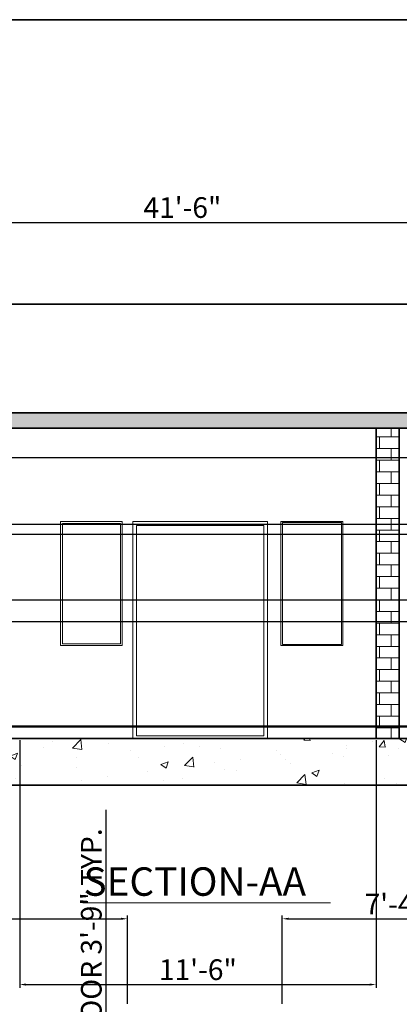
# Model space of a CAD drawing. Units: inches. Extents: x 2257 to 3678, y 834 to 1975.
# Tile 10 of 16: x 3191 to 3338, y 1594 to 1975. Entities that reach past the tile are written whole.
import ezdxf

# ---------------------------------------------------------------- set-up
doc = ezdxf.new("R2010")
doc.units = ezdxf.units.IN
for name, color, linetype, lineweight in [('A-ANNO-DIMS', 2, 'Continuous', 18), ('A-ANNO-TEXT', 7, 'Continuous', 18), ('A-ANNO-TTLB', 7, 'Continuous', 35), ('A-ELEV-DOOR', 3, 'Continuous', 18), ('A-ELEV-GLAZ', 4, 'Continuous', 18), ('A-SECT', 7, 'Continuous', 35), ('A-SECT-BRCK-PATT', 252, 'Continuous', 13), ('A-SECT-CONC-PATT', 252, 'Continuous', 13)]:
    doc.layers.add(name, color=color, linetype=linetype, lineweight=lineweight)
doc.styles.get("Standard").update_dxf_attribs({"font": 'arial.ttf'})
doc.dimstyles.new('ISO-25', dxfattribs={"dimtxt": 8, "dimasz": 2.5, "dimexe": 1.25, "dimexo": 0.625, "dimtad": 1, "dimdec": 0, "dimlunit": 3, "dimtxsty": 'Standard', "dimcen": 2.5, "dimadec": 0, "dimazin": 0, "dimtfac": 1, "dimtdec": 0, "dimtmove": 0, "dimatfit": 3, "dimfxl": 1, "dimarcsym": 0})

# ---------------------------------------------------------------- blocks, each defined once
blk = doc.blocks.new('*D62')
at = {"layer": 'A-ANNO-DIMS', "color": 0, "lineweight": -2, "transparency": 16777216}
for p, q in [((3224.23, 1485.58), (3224.23, 1669.32)), ((3218.11, 1485.58), (3225.48, 1485.58)), ((3224.23, 1443.08), (3224.23, 1483.08)), ((3218.11, 1440.58), (3225.48, 1440.58))]:
    blk.add_line(p, q, dxfattribs=at)
at = {"layer": 'A-ANNO-DIMS', "color": 0, "transparency": 16777216}
for points in [[(3223.82, 1483.08), (3224.65, 1483.08), (3224.23, 1485.58)], [(3223.82, 1443.08), (3224.65, 1443.08), (3224.23, 1440.58)]]:
    blk.add_solid(points, dxfattribs=at)
at = {"layer": 'Defpoints', "color": 0, "transparency": 16777216}
for p in [(3217.48, 1485.58), (3224.23, 1485.58), (3217.48, 1440.58)]:
    blk.add_point(p, dxfattribs=at)
at = {"layer": 'A-ANNO-DIMS', "color": 0, "transparency": 16777216, "insert": (3219.47, 1578.7), "char_height": 8, "attachment_point": 5, "rotation": 90}
blk.add_mtext('REAR BEDROOM DOOR 3\'-9" TYP.', dxfattribs=at)
blk = doc.blocks.new('*D109')
at = {"layer": 'A-ANNO-DIMS', "color": 0, "lineweight": -2, "transparency": 16777216}
for p, q in [((3112.29, 1594.2), (3112.29, 1628.38)), ((3114.79, 1627.13), (3229.89, 1627.13)), ((3232.39, 1594.2), (3232.39, 1628.38))]:
    blk.add_line(p, q, dxfattribs=at)
at = {"layer": 'A-ANNO-DIMS', "color": 0, "transparency": 16777216}
for points in [[(3114.79, 1627.54), (3114.79, 1626.71), (3112.29, 1627.13)], [(3229.89, 1627.54), (3229.89, 1626.71), (3232.39, 1627.13)]]:
    blk.add_solid(points, dxfattribs=at)
at = {"layer": 'Defpoints', "color": 0, "transparency": 16777216}
for p in [(3232.39, 1627.13), (3112.29, 1593.58), (3232.39, 1593.58)]:
    blk.add_point(p, dxfattribs=at)
at = {"layer": 'A-ANNO-DIMS', "color": 0, "transparency": 16777216, "insert": (3172.34, 1631.84), "char_height": 8, "attachment_point": 5}
blk.add_mtext('10\'-0"', dxfattribs=at)
blk = doc.blocks.new('*D110')
at = {"layer": 'A-ANNO-DIMS', "color": 0, "lineweight": -2, "transparency": 16777216}
for p, q in [((3292.39, 1594.2), (3292.39, 1628.38)), ((3294.89, 1627.13), (3377.71, 1627.13)), ((3380.21, 1594.2), (3380.21, 1628.38))]:
    blk.add_line(p, q, dxfattribs=at)
at = {"layer": 'A-ANNO-DIMS', "color": 0, "transparency": 16777216}
for points in [[(3294.89, 1627.54), (3294.89, 1626.71), (3292.39, 1627.13)], [(3377.71, 1627.54), (3377.71, 1626.71), (3380.21, 1627.13)]]:
    blk.add_solid(points, dxfattribs=at)
at = {"layer": 'Defpoints', "color": 0, "transparency": 16777216}
for p in [(3380.21, 1627.13), (3292.39, 1593.58), (3380.21, 1593.58)]:
    blk.add_point(p, dxfattribs=at)
at = {"layer": 'A-ANNO-DIMS', "color": 0, "transparency": 16777216, "insert": (3336.3, 1631.75), "char_height": 8, "attachment_point": 5}
blk.add_mtext('7\'-4"', dxfattribs=at)
blk = doc.blocks.new('*D133')
at = {"layer": 'A-ANNO-DIMS', "color": 0, "lineweight": -2, "transparency": 16777216}
for p, q in [((3004.7, 1865.47), (3004.7, 1897.74)), ((3502.7, 1865.47), (3502.7, 1897.74)), ((3007.2, 1896.49), (3500.2, 1896.49))]:
    blk.add_line(p, q, dxfattribs=at)
at = {"layer": 'A-ANNO-DIMS', "color": 0, "transparency": 16777216}
for points in [[(3007.2, 1896.91), (3007.2, 1896.07), (3004.7, 1896.49)], [(3500.2, 1896.91), (3500.2, 1896.07), (3502.7, 1896.49)]]:
    blk.add_solid(points, dxfattribs=at)
at = {"layer": 'Defpoints', "color": 0, "transparency": 16777216}
for p in [(3502.7, 1896.49), (3004.7, 1864.84), (3502.7, 1864.84)]:
    blk.add_point(p, dxfattribs=at)
at = {"layer": 'A-ANNO-DIMS', "color": 0, "transparency": 16777216, "insert": (3253.7, 1901.2), "char_height": 8, "attachment_point": 5}
blk.add_mtext('41\'-6"', dxfattribs=at)
blk = doc.blocks.new('*D136')
at = {"layer": 'A-ANNO-DIMS', "color": 0, "lineweight": -2, "transparency": 16777216}
for p, q in [((3190.7, 1696.22), (3190.7, 1600.44)), ((3328.7, 1696.22), (3328.7, 1600.44)), ((3193.2, 1601.69), (3326.2, 1601.69))]:
    blk.add_line(p, q, dxfattribs=at)
at = {"layer": 'A-ANNO-DIMS', "color": 0, "transparency": 16777216}
for points in [[(3193.2, 1602.1), (3193.2, 1601.27), (3190.7, 1601.69)], [(3326.2, 1602.1), (3326.2, 1601.27), (3328.7, 1601.69)]]:
    blk.add_solid(points, dxfattribs=at)
at = {"layer": 'Defpoints', "color": 0, "transparency": 16777216}
for p in [(3190.7, 1696.84), (3328.7, 1696.84), (3328.7, 1601.69)]:
    blk.add_point(p, dxfattribs=at)
at = {"layer": 'A-ANNO-DIMS', "color": 0, "transparency": 16777216, "insert": (3259.7, 1606.4), "char_height": 8, "attachment_point": 5}
blk.add_mtext('11\'-6"', dxfattribs=at)
blk = doc.blocks.new('*D145')
at = {"layer": 'A-ANNO-DIMS', "color": 0, "lineweight": -2, "transparency": 16777216}
for p, q in [((3353.28, 1805.46), (2971.8, 1805.46)), ((2973.05, 1782.13), (2973.05, 1802.96)), ((3353.28, 1779.63), (2971.8, 1779.63))]:
    blk.add_line(p, q, dxfattribs=at)
at = {"layer": 'A-ANNO-DIMS', "color": 0, "transparency": 16777216}
for points in [[(2972.63, 1802.96), (2973.47, 1802.96), (2973.05, 1805.46)], [(2972.63, 1782.13), (2973.47, 1782.13), (2973.05, 1779.63)]]:
    blk.add_solid(points, dxfattribs=at)
at = {"layer": 'Defpoints', "color": 0, "transparency": 16777216}
for p in [(2973.05, 1805.46), (3353.91, 1805.46), (3353.91, 1779.63)]:
    blk.add_point(p, dxfattribs=at)
at = {"layer": 'A-ANNO-DIMS', "color": 0, "transparency": 16777216, "insert": (2968.41, 1792.54), "char_height": 8, "attachment_point": 5, "rotation": 90}
blk.add_mtext('2\'-2"', dxfattribs=at)
blk = doc.blocks.new('*D146')
at = {"layer": 'A-ANNO-DIMS', "color": 0, "lineweight": -2, "transparency": 16777216}
for p, q in [((2973.05, 1703.73), (2973.05, 1747.39)), ((3353.28, 1701.23), (2971.8, 1701.23)), ((2973.05, 1696.7), (2973.05, 1701.23)), ((3353.28, 1696.7), (2971.8, 1696.7)), ((2973.05, 1694.2), (2973.05, 1691.7))]:
    blk.add_line(p, q, dxfattribs=at)
at = {"layer": 'A-ANNO-DIMS', "color": 0, "transparency": 16777216}
for points in [[(2972.63, 1703.73), (2973.47, 1703.73), (2973.05, 1701.23)], [(2972.63, 1694.2), (2973.47, 1694.2), (2973.05, 1696.7)]]:
    blk.add_solid(points, dxfattribs=at)
at = {"layer": 'Defpoints', "color": 0, "transparency": 16777216}
for p in [(2973.05, 1701.23), (3353.91, 1701.23), (3353.91, 1696.7)]:
    blk.add_point(p, dxfattribs=at)
at = {"layer": 'A-ANNO-DIMS', "color": 0, "transparency": 16777216, "insert": (2968.29, 1726.81), "char_height": 8, "attachment_point": 5, "rotation": 90}
blk.add_mtext('0\'-4 1/2"', dxfattribs=at)
blk = doc.blocks.new('*D148')
at = {"layer": 'A-ANNO-DIMS', "color": 0, "lineweight": -2, "transparency": 16777216}
for p, q in [((3375.03, 1775.78), (2971.8, 1775.78)), ((2973.05, 1744.52), (2973.05, 1773.28)), ((3375.03, 1742.02), (2971.8, 1742.02))]:
    blk.add_line(p, q, dxfattribs=at)
at = {"layer": 'A-ANNO-DIMS', "color": 0, "transparency": 16777216}
for points in [[(2972.63, 1773.28), (2973.47, 1773.28), (2973.05, 1775.78)], [(2972.63, 1744.52), (2973.47, 1744.52), (2973.05, 1742.02)]]:
    blk.add_solid(points, dxfattribs=at)
at = {"layer": 'Defpoints', "color": 0, "transparency": 16777216}
for p in [(2973.05, 1775.78), (3375.66, 1775.78), (3375.66, 1742.02)]:
    blk.add_point(p, dxfattribs=at)
at = {"layer": 'A-ANNO-DIMS', "color": 0, "transparency": 16777216, "insert": (2968.34, 1758.9), "char_height": 8, "attachment_point": 5, "rotation": 90}
blk.add_mtext('2\'-10"', dxfattribs=at)
blk = doc.blocks.new('*D149')
at = {"layer": 'A-ANNO-DIMS', "color": 0, "lineweight": -2, "transparency": 16777216}
for p, q in [((3417.18, 1750.35), (2971.8, 1750.35)), ((2973.05, 1704.19), (2973.05, 1747.85)), ((3417.18, 1701.69), (2971.8, 1701.69))]:
    blk.add_line(p, q, dxfattribs=at)
at = {"layer": 'A-ANNO-DIMS', "color": 0, "transparency": 16777216}
for points in [[(2972.63, 1747.85), (2973.47, 1747.85), (2973.05, 1750.35)], [(2972.63, 1704.19), (2973.47, 1704.19), (2973.05, 1701.69)]]:
    blk.add_solid(points, dxfattribs=at)
at = {"layer": 'Defpoints', "color": 0, "transparency": 16777216}
for p in [(2973.05, 1750.35), (3417.8, 1750.35), (3417.8, 1701.69)]:
    blk.add_point(p, dxfattribs=at)
at = {"layer": 'A-ANNO-DIMS', "color": 0, "transparency": 16777216, "insert": (2968.29, 1726.02), "char_height": 8, "attachment_point": 5, "rotation": 90}
blk.add_mtext('4\'-0 1/2"', dxfattribs=at)

msp = doc.modelspace()

# ---------------------------------------------------------------- hatches: boundary and pattern name
at = {"layer": 'A-SECT-BRCK-PATT'}
h = msp.add_hatch(dxfattribs=at)
h.set_pattern_fill('BRICK', color=256, scale=0.708661, style=0)
h.paths.add_polyline_path([(3328.7, 1696.84), (3337.7, 1696.84), (3337.7, 1816.84), (3328.7, 1816.84)])
at = {"layer": 'A-SECT-CONC-PATT'}
h = msp.add_hatch(dxfattribs=at)
h.set_pattern_fill('AR-CONC', color=256, scale=0.035, style=0)
h.paths.add_polyline_path([(3004.7, 1816.84), (3502.7, 1816.84), (3502.7, 1822.84), (3004.7, 1822.84)])
h = msp.add_hatch(dxfattribs=at)
h.set_pattern_fill('AR-CONC', color=256, scale=0.16, style=0)
h.paths.add_polyline_path([(3004.7, 1678.84), (3502.7, 1678.84), (3502.7, 1696.84), (3004.7, 1696.84)])

# ---------------------------------------------------------------- linework, layer by layer
at = {"layer": 'A-ANNO-TEXT'}
msp.add_line((3215.12, 1633.34), (3311.06, 1633.34), dxfattribs=at)
at = {"layer": 'A-ANNO-TTLB'}
msp.add_lwpolyline([(2257.38, 1974.9), (3677.96, 1974.9), (3677.96, 849.42), (2257.38, 849.42)], close=True, dxfattribs=at)
at = {"layer": 'A-ELEV-DOOR'}
for p, q in [((3234.47, 1780.84), (3234.47, 1696.84)), ((3286.61, 1780.84), (3234.47, 1780.84)), ((3286.61, 1780.84), (3286.61, 1696.84))]:
    msp.add_line(p, q, dxfattribs=at)
msp.add_lwpolyline([(3235.96, 1779.24), (3285.29, 1779.24), (3285.29, 1697.9), (3235.96, 1697.9)], close=True, dxfattribs=at)
at = {"layer": 'A-ELEV-GLAZ'}
for p, q in [((3206.45, 1780.84), (3206.45, 1732.84)), ((3230.45, 1780.84), (3206.45, 1780.84)), ((3230.45, 1780.84), (3230.45, 1732.84)), ((3291.87, 1780.84), (3291.87, 1732.84)), ((3315.87, 1780.84), (3291.87, 1780.84)), ((3315.87, 1780.84), (3315.87, 1732.84)), ((3230.45, 1732.84), (3206.45, 1732.84)), ((3315.87, 1732.84), (3291.87, 1732.84))]:
    msp.add_line(p, q, dxfattribs=at)
for points in [[(3207.28, 1779.99), (3229.75, 1779.99), (3229.75, 1733.49), (3207.28, 1733.49)], [(3292.45, 1780.37), (3315.31, 1780.37), (3315.31, 1733.21), (3292.45, 1733.21)]]:
    msp.add_lwpolyline(points, close=True, dxfattribs=at)
at = {"layer": 'A-SECT'}
for p, q in [((3502.7, 1864.84), (3004.7, 1864.84)), ((3502.7, 1822.84), (3004.7, 1822.84)), ((3196.31, 1816.84), (3004.7, 1816.84)), ((3502.7, 1816.84), (3196.31, 1816.84)), ((3328.7, 1696.84), (3328.7, 1816.84)), ((3337.7, 1696.84), (3337.7, 1816.84)), ((3502.7, 1696.84), (3004.7, 1696.84)), ((3502.7, 1678.84), (3004.7, 1678.84))]:
    msp.add_line(p, q, dxfattribs=at)

# ---------------------------------------------------------------- texts
at = {"layer": 'A-ANNO-TEXT', "insert": (3215.42, 1647.02), "char_height": 11, "attachment_point": 1}
msp.add_mtext_dynamic_manual_height_columns('SECTION-AA', width=195.7365, gutter_width=12.5, heights=[0], dxfattribs=at)

# ---------------------------------------------------------------- dimensions: what is measured, and where the dimension line sits
at = {"layer": 'A-ANNO-DIMS'}
for base, p1, p2, picture, middle in [((3502.7, 1896.49), (3004.7, 1864.84), (3502.7, 1864.84), '*D133', (3253.7, 1901.2)), ((3328.7, 1601.69), (3190.7, 1696.84), (3328.7, 1696.84), '*D136', (3259.7, 1606.4)), ((3232.39, 1627.13), (3112.29, 1593.58), (3232.39, 1593.58), '*D109', (3172.34, 1631.84)), ((3380.21, 1627.13), (3292.39, 1593.58), (3380.21, 1593.58), '*D110', (3336.3, 1631.75))]:
    dim = msp.add_linear_dim(base=base, p1=p1, p2=p2, dimstyle='ISO-25', override={"dimdec": 1, "dimlfac": 1, "dimrnd": 0, "dimzin": 1, "dimdsep": 46, "dimlunit": 4, "dimfrac": 2}, dxfattribs=at)
    dim.commit()
    dim.dimension.update_dxf_attribs({"geometry": picture, "text_midpoint": middle})
for base, p1, p2, picture, middle in [((2973.05, 1805.46), (3353.91, 1779.63), (3353.91, 1805.46), '*D145', (2968.41, 1792.54)), ((2973.05, 1775.78), (3375.66, 1742.02), (3375.66, 1775.78), '*D148', (2968.34, 1758.9)), ((2973.05, 1750.35), (3417.8, 1701.69), (3417.8, 1750.35), '*D149', (2968.29, 1726.02)), ((2973.05, 1701.23), (3353.91, 1696.7), (3353.91, 1701.23), '*D146', (2968.29, 1726.81))]:
    dim = msp.add_linear_dim(base=base, p1=p1, p2=p2, angle=90, dimstyle='ISO-25', override={"dimdec": 1, "dimlfac": 1, "dimrnd": 0, "dimzin": 1, "dimdsep": 46, "dimlunit": 4, "dimfrac": 2}, dxfattribs=at)
    dim.commit()
    dim.dimension.update_dxf_attribs({"geometry": picture, "text_midpoint": middle})
dim = msp.add_linear_dim(base=(3224.23, 1485.58), p1=(3217.48, 1440.58), p2=(3217.48, 1485.58), angle=90, text='REAR BEDROOM DOOR <> TYP.', dimstyle='ISO-25', override={"dimdec": 1, "dimlfac": 1, "dimrnd": 0, "dimzin": 1, "dimdsep": 46, "dimlunit": 4, "dimfrac": 2}, dxfattribs=at)
dim.commit()
dim.dimension.update_dxf_attribs({"geometry": '*D62', "text_midpoint": (3219.47, 1578.7)})

doc.saveas('drawing.dxf')
